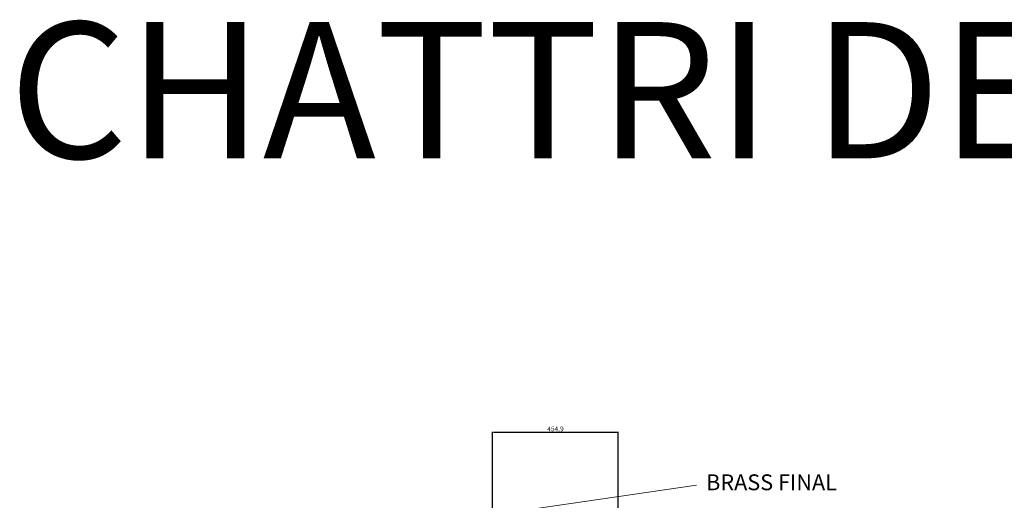
# Model space of a CAD drawing. Units: millimetres. Extents: x 498 to 8860, y -426 to 8717.
# Tile 7 of 9: x 683 to 4247, y 6976 to 8717. Entities that reach past the tile are written whole.
import ezdxf

# ---------------------------------------------------------------- set-up
doc = ezdxf.new("R2010")
doc.units = ezdxf.units.MM
doc.layers.add('A-ANNO-DIMS', color=2, linetype='Continuous', lineweight=18)
doc.layers.add('A-ANNO-TEXT', color=3, linetype='Continuous', lineweight=18)
doc.styles.get("Standard").update_dxf_attribs({"font": 'arial.ttf'})
doc.dimstyles.new('ISO-25', dxfattribs={"dimtxt": 17.5, "dimasz": 2.5, "dimexe": 1.25, "dimexo": 0.625, "dimtad": 1, "dimdec": 0, "dimtxsty": 'Standard', "dimcen": 2.5, "dimadec": 0, "dimazin": 0, "dimtfac": 1, "dimtdec": 0, "dimtmove": 0, "dimatfit": 3, "dimfxl": 1, "dimarcsym": 0})

# ---------------------------------------------------------------- blocks, each defined once
blk = doc.blocks.new('*D49')
at = {"layer": 'A-ANNO-DIMS', "color": 0, "lineweight": -2, "transparency": 16777216}
for p, q in [((2394.7, 5875.8), (2394.7, 7224.4)), ((2397.2, 7223.1), (2847.1, 7223.1)), ((2849.6, 5664.6), (2849.6, 7224.4))]:
    blk.add_line(p, q, dxfattribs=at)
at = {"layer": 'A-ANNO-DIMS', "color": 0, "transparency": 16777216}
for points in [[(2397.2, 7223.5), (2397.2, 7222.7), (2394.7, 7223.1)], [(2847.1, 7223.5), (2847.1, 7222.7), (2849.6, 7223.1)]]:
    blk.add_solid(points, dxfattribs=at)
at = {"layer": 'Defpoints', "color": 0, "transparency": 16777216}
for p in [(2849.6, 7223.1), (2394.7, 5875.2), (2849.6, 5664)]:
    blk.add_point(p, dxfattribs=at)
at = {"layer": 'A-ANNO-DIMS', "color": 0, "transparency": 16777216, "insert": (2622.2, 7232.7), "char_height": 17.5, "attachment_point": 5}
blk.add_mtext('454.9', dxfattribs=at)

msp = doc.modelspace()

# ---------------------------------------------------------------- linework, layer by layer
at = {"layer": 'A-ANNO-TEXT'}
msp.add_lwpolyline([(1849.694, 6844.528), (3132.176, 7031.12)], dxfattribs=at)

# ---------------------------------------------------------------- texts
for s, height, p in [('CHATTRI DETAIL', 493.33964, (643.54, 8214.558)), ('BRASS FINAL', 57.54038, (3167.376, 7012.887))]:
    msp.add_text(s, height=height, dxfattribs=at).set_placement(p)

# ---------------------------------------------------------------- dimensions: what is measured, and where the dimension line sits
at = {"layer": 'A-ANNO-DIMS'}
dim = msp.add_linear_dim(base=(2849.644, 7223.12), p1=(2394.726, 5875.163), p2=(2849.644, 5663.993), dimstyle='ISO-25', override={"dimdec": 1, "dimlfac": 1, "dimrnd": 0, "dimzin": 0, "dimdsep": 46, "dimlunit": 2}, dxfattribs=at)
dim.commit()
dim.dimension.update_dxf_attribs({"geometry": '*D49', "text_midpoint": (2622.185, 7232.68)})

doc.saveas('drawing.dxf')
